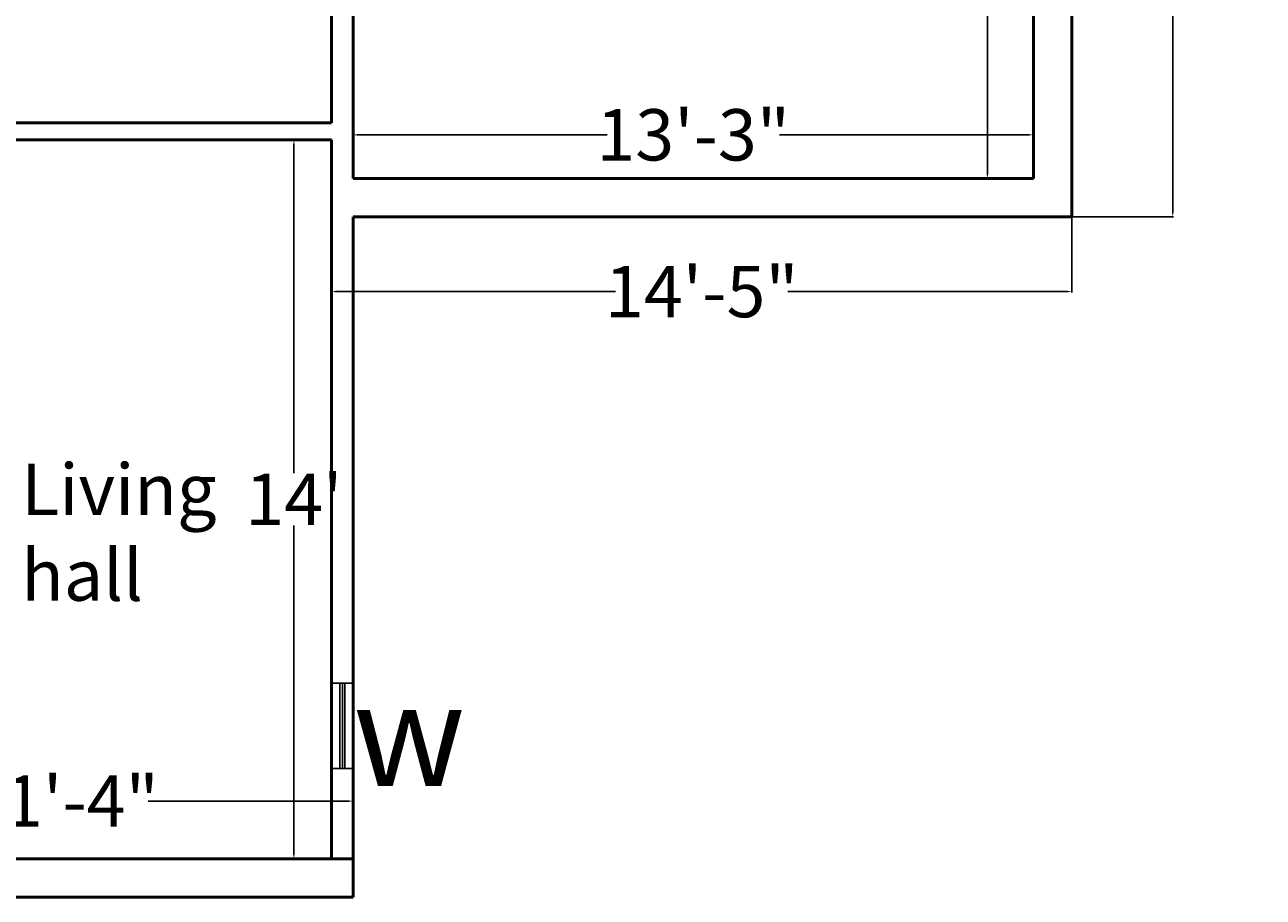
# Model space of a CAD drawing. Units: inches. Extents: x 409 to 7572, y 7 to 725.
# Tile 25 of 38: x 4623 to 4913, y 157 to 360. Entities that reach past the tile are written whole.
import ezdxf

# ---------------------------------------------------------------- set-up
doc = ezdxf.new("R2010")
doc.units = ezdxf.units.IN
doc.header["$MEASUREMENT"] = 0
for name, color, linetype, lineweight in [('A-ANNO-DIMS', 2, 'Continuous', 18), ('A-ANNO-SYMB', 3, 'Continuous', 25), ('A-AREA-IDEN', 7, 'Continuous', 25), ('A-GLAZ', 4, 'Continuous', 25), ('A-WALL', 7, 'Continuous', 50)]:
    doc.layers.add(name, color=color, linetype=linetype, lineweight=lineweight)
doc.styles.get("Standard").update_dxf_attribs({"font": 'arial.ttf'})
doc.dimstyles.get("Standard").update_dxf_attribs({"dimtxt": 2, "dimasz": 1, "dimexe": 0.18, "dimexo": 0.0625, "dimgap": 0.09, "dimtad": 0, "dimtih": 1, "dimtoh": 1, "dimdec": 0, "dimzin": 0, "dimdsep": 46, "dimlunit": 3, "dimtxsty": 'Standard', "dimcen": 0.09, "dimadec": 0, "dimazin": 0, "dimtfac": 1, "dimtdec": 0, "dimtofl": 0, "dimtmove": 0, "dimatfit": 3, "dimfxl": 1, "dimtolj": 1, "dimtzin": 0, "dimarcsym": 0})

# ---------------------------------------------------------------- blocks, each defined once
blk = doc.blocks.new('*D103')
at = {"layer": 'A-ANNO-DIMS', "color": 0, "lineweight": -2, "transparency": 16777216}
for p, q in [((4858.88, 444.53), (4848, 444.53)), ((4848.18, 443.53), (4848.18, 390.75)), ((4848.18, 325.53), (4848.18, 378.31)), ((4858.88, 324.53), (4848, 324.53))]:
    blk.add_line(p, q, dxfattribs=at)
at = {"layer": 'A-ANNO-DIMS', "color": 0, "transparency": 16777216}
for points in [[(4848.01, 443.53), (4848.34, 443.53), (4848.18, 444.53)], [(4848.01, 325.53), (4848.34, 325.53), (4848.18, 324.53)]]:
    blk.add_solid(points, dxfattribs=at)
at = {"layer": 'DEFPOINTS', "color": 0, "transparency": 16777216}
for p in [(4848.18, 444.53), (4858.94, 444.53), (4858.94, 324.53)]:
    blk.add_point(p, dxfattribs=at)
at = {"layer": 'A-ANNO-DIMS', "color": 0, "transparency": 16777216, "insert": (4848.18, 384.53), "char_height": 2, "attachment_point": 5}
blk.add_mtext("\\A1;{\\H6x;10'}", dxfattribs=at)
blk = doc.blocks.new('*D94')
at = {"layer": 'A-ANNO-DIMS', "color": 0, "lineweight": -2, "transparency": 16777216}
for p, q in [((4699.94, 324.59), (4699.94, 334.9)), ((4700.94, 334.72), (4759.3, 334.72)), ((4857.94, 334.72), (4799.58, 334.72)), ((4858.94, 324.59), (4858.94, 334.9))]:
    blk.add_line(p, q, dxfattribs=at)
at = {"layer": 'A-ANNO-DIMS', "color": 0, "transparency": 16777216}
for points in [[(4700.94, 334.88), (4700.94, 334.55), (4699.94, 334.72)], [(4857.94, 334.88), (4857.94, 334.55), (4858.94, 334.72)]]:
    blk.add_solid(points, dxfattribs=at)
at = {"layer": 'DEFPOINTS', "color": 0, "transparency": 16777216}
for p in [(4699.94, 334.72), (4699.94, 324.53), (4858.94, 324.53)]:
    blk.add_point(p, dxfattribs=at)
at = {"layer": 'A-ANNO-DIMS', "color": 0, "transparency": 16777216, "insert": (4779.44, 334.72), "char_height": 2, "attachment_point": 5}
blk.add_mtext('\\A1;{\\H6x;13\'-3"}', dxfattribs=at)
blk = doc.blocks.new('*D95')
at = {"layer": 'A-ANNO-DIMS', "color": 0, "lineweight": -2, "transparency": 16777216}
for p, q in [((4694.88, 333.53), (4685.95, 333.53)), ((4686.13, 332.53), (4686.13, 255.65)), ((4686.13, 166.53), (4686.13, 243.42)), ((4694.88, 165.53), (4685.95, 165.53))]:
    blk.add_line(p, q, dxfattribs=at)
at = {"layer": 'A-ANNO-DIMS', "color": 0, "transparency": 16777216}
for points in [[(4685.96, 332.53), (4686.29, 332.53), (4686.13, 333.53)], [(4685.96, 166.53), (4686.29, 166.53), (4686.13, 165.53)]]:
    blk.add_solid(points, dxfattribs=at)
at = {"layer": 'DEFPOINTS', "color": 0, "transparency": 16777216}
for p in [(4694.94, 333.53), (4686.13, 165.53), (4694.94, 165.53)]:
    blk.add_point(p, dxfattribs=at)
at = {"layer": 'A-ANNO-DIMS', "color": 0, "transparency": 16777216, "insert": (4686.13, 249.53), "char_height": 2, "attachment_point": 5}
blk.add_mtext("\\A1;{\\H6x;14'}", dxfattribs=at)
blk = doc.blocks.new('*D96')
at = {"layer": 'A-ANNO-DIMS', "color": 0, "lineweight": -2, "transparency": 16777216}
for p, q in [((4563.94, 165.59), (4563.94, 179.18)), ((4564.94, 179), (4611.8, 179)), ((4698.94, 179), (4652.08, 179)), ((4699.94, 165.59), (4699.94, 179.18))]:
    blk.add_line(p, q, dxfattribs=at)
at = {"layer": 'A-ANNO-DIMS', "color": 0, "transparency": 16777216}
for points in [[(4564.94, 179.16), (4564.94, 178.83), (4563.94, 179)], [(4698.94, 179.16), (4698.94, 178.83), (4699.94, 179)]]:
    blk.add_solid(points, dxfattribs=at)
at = {"layer": 'DEFPOINTS', "color": 0, "transparency": 16777216}
for p in [(4699.94, 179), (4563.94, 165.53), (4699.94, 165.53)]:
    blk.add_point(p, dxfattribs=at)
at = {"layer": 'A-ANNO-DIMS', "color": 0, "transparency": 16777216, "insert": (4631.94, 179), "char_height": 2, "attachment_point": 5}
blk.add_mtext('\\A1;{\\H6x;11\'-4"}', dxfattribs=at)
blk = doc.blocks.new('*D120')
at = {"layer": 'A-ANNO-DIMS', "color": 0, "lineweight": -2, "transparency": 16777216}
for p, q in [((4868, 672.53), (4891.69, 672.53)), ((4891.51, 671.53), (4891.51, 500.86)), ((4891.51, 316.53), (4891.51, 488.43)), ((4868, 315.53), (4891.69, 315.53))]:
    blk.add_line(p, q, dxfattribs=at)
at = {"layer": 'A-ANNO-DIMS', "color": 0, "transparency": 16777216}
for points in [[(4891.34, 671.53), (4891.67, 671.53), (4891.51, 672.53)], [(4891.34, 316.53), (4891.67, 316.53), (4891.51, 315.53)]]:
    blk.add_solid(points, dxfattribs=at)
at = {"layer": 'DEFPOINTS', "color": 0, "transparency": 16777216}
for p in [(4867.94, 672.53), (4891.51, 672.53), (4867.94, 315.53)]:
    blk.add_point(p, dxfattribs=at)
at = {"layer": 'A-ANNO-DIMS', "color": 0, "transparency": 16777216, "insert": (4891.51, 494.65), "char_height": 2, "attachment_point": 5}
blk.add_mtext('\\A1;{\\H6x;29\'-9"}', dxfattribs=at)
blk = doc.blocks.new('*D119')
at = {"layer": 'A-ANNO-DIMS', "color": 0, "lineweight": -2, "transparency": 16777216}
for p, q in [((4694.94, 315.37), (4694.94, 297.9)), ((4867.94, 315.37), (4867.94, 297.9)), ((4695.94, 298.08), (4761.3, 298.08)), ((4866.94, 298.08), (4801.58, 298.08))]:
    blk.add_line(p, q, dxfattribs=at)
at = {"layer": 'A-ANNO-DIMS', "color": 0, "transparency": 16777216}
for points in [[(4695.94, 298.25), (4695.94, 297.92), (4694.94, 298.08)], [(4866.94, 298.25), (4866.94, 297.92), (4867.94, 298.08)]]:
    blk.add_solid(points, dxfattribs=at)
at = {"layer": 'DEFPOINTS', "color": 0, "transparency": 16777216}
for p in [(4694.94, 315.43), (4867.94, 315.43), (4867.94, 298.08)]:
    blk.add_point(p, dxfattribs=at)
at = {"layer": 'A-ANNO-DIMS', "color": 0, "transparency": 16777216, "insert": (4781.44, 298.08), "char_height": 2, "attachment_point": 5}
blk.add_mtext('\\A1;{\\H6x;14\'-5"}', dxfattribs=at)
blk = doc.blocks.new('WIN-20')
for p, q in [((2103.48, 182.68), (2083.54, 182.68)), ((2103.48, 182.13), (2083.54, 182.13)), ((2103.48, 181.57), (2083.54, 181.57))]:
    blk.add_line(p, q)
blk.add_lwpolyline([(2103.48, 179.64), (2083.54, 179.64), (2083.54, 184.62), (2103.48, 184.62)], close=True)

msp = doc.modelspace()

# ---------------------------------------------------------------- linework, layer by layer
at = {"layer": 'A-WALL'}
for p, q in [((4867.94, 315.53), (4867.94, 672.53)), ((4694.94, 525.53), (4694.94, 337.53)), ((4694.94, 489.53), (4694.94, 337.53)), ((4699.94, 444.53), (4699.94, 324.53)), ((4858.94, 324.53), (4858.94, 444.53)), ((4609, 337.53), (4694.94, 337.53)), ((4609, 333.53), (4694.94, 333.53)), ((4694.94, 333.53), (4694.94, 165.53)), ((4694.94, 333.53), (4694.94, 165.53)), ((4858.94, 324.53), (4699.94, 324.53)), ((4867.94, 315.53), (4699.94, 315.53)), ((4699.94, 315.53), (4699.94, 165.53)), ((4563.94, 165.53), (4699.94, 165.53)), ((4699.94, 165.53), (4699.94, 156.53)), ((4325.94, 156.53), (4699.94, 156.53))]:
    msp.add_line(p, q, dxfattribs=at)

# ---------------------------------------------------------------- block references
at = {"layer": 'A-GLAZ', "rotation": 89.99999999999451}
msp.add_blockref('WIN-20', (4879.58, -1896.94), dxfattribs=at)

# ---------------------------------------------------------------- texts
at = {"layer": 'A-ANNO-SYMB', "insert": (4699.94, 206.54), "char_height": 24, "attachment_point": 1}
msp.add_mtext_dynamic_manual_height_columns('w', width=18.2582, gutter_width=1, heights=[0], dxfattribs=at)
at = {"layer": 'A-AREA-IDEN', "insert": (4622.41, 257.83), "char_height": 12, "attachment_point": 1}
msp.add_mtext_dynamic_manual_height_columns('Living hall', width=58.8843, gutter_width=1, heights=[0], dxfattribs=at)

# ---------------------------------------------------------------- dimensions: what is measured, and where the dimension line sits
at = {"layer": 'A-ANNO-DIMS'}
dim = msp.add_linear_dim(base=(4891.51, 672.53), p1=(4867.94, 315.53), p2=(4867.94, 672.53), angle=90, text='{\\H6x;<>}', dimstyle='Standard', override={"dimclrd": 0, "dimclre": 0, "dimclrt": 0}, dxfattribs=at)
dim.commit()
dim.dimension.update_dxf_attribs({"geometry": '*D120', "text_midpoint": (4891.51, 494.65), "dimtype": 160})
for base, p1, p2, picture, middle in [((4848.18, 444.53), (4858.94, 324.53), (4858.94, 444.53), '*D103', (4848.18, 384.53)), ((4686.13, 165.53), (4694.94, 333.53), (4694.94, 165.53), '*D95', (4686.13, 249.53))]:
    dim = msp.add_linear_dim(base=base, p1=p1, p2=p2, angle=90, text='{\\H6x;<>}', dimstyle='Standard', override={"dimclrd": 0, "dimclre": 0, "dimclrt": 0}, dxfattribs=at)
    dim.commit()
    dim.dimension.update_dxf_attribs({"geometry": picture, "text_midpoint": middle})
for base, p1, p2, picture, middle in [((4699.94, 334.72), (4858.94, 324.53), (4699.94, 324.53), '*D94', (4779.44, 334.72)), ((4867.94, 298.08), (4694.94, 315.43), (4867.94, 315.43), '*D119', (4781.44, 298.08)), ((4699.94, 179), (4563.94, 165.53), (4699.94, 165.53), '*D96', (4631.94, 179))]:
    dim = msp.add_linear_dim(base=base, p1=p1, p2=p2, text='{\\H6x;<>}', dimstyle='Standard', override={"dimclrd": 0, "dimclre": 0, "dimclrt": 0}, dxfattribs=at)
    dim.commit()
    dim.dimension.update_dxf_attribs({"geometry": picture, "text_midpoint": middle})

doc.saveas('drawing.dxf')
